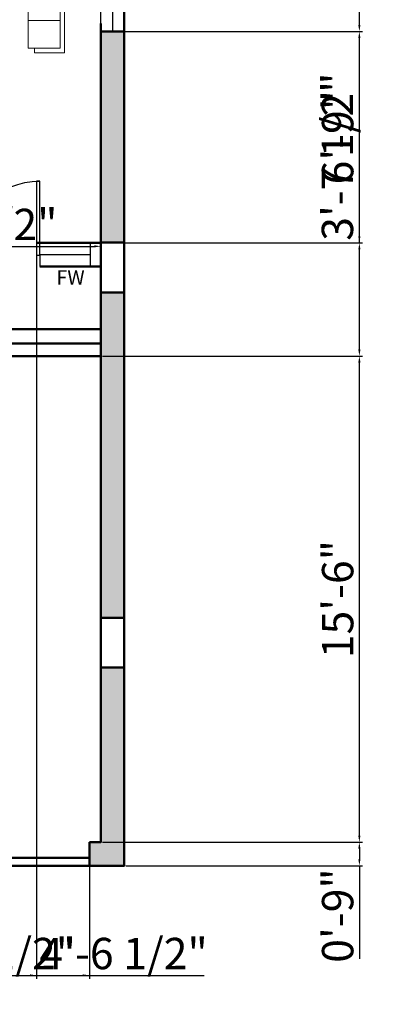
# Model space of a CAD drawing. Units: inches. Extents: x 2063 to 3370, y 2091 to 2971.
# Tile 2 of 14: x 2345 to 2486, y 2091 to 2468. Entities that reach past the tile are written whole.
import ezdxf

# ---------------------------------------------------------------- set-up
doc = ezdxf.new("R2010")
doc.units = ezdxf.units.IN
for name, color, linetype, lineweight in [('A-ANNO-DIMS', 2, 'Continuous', 18), ('A-ANNO-TEXT', 7, 'Continuous', 18), ('A-COLS', 7, 'Continuous', 50), ('A-DOOR', 4, 'Continuous', 25), ('A-FURN', 8, 'Continuous', 18), ('A-GLAZ', 131, 'Continuous', 25), ('A-WALL', 7, 'Continuous', 50), ('A-WALL-PATT', 8, 'Continuous', 13)]:
    doc.layers.add(name, color=color, linetype=linetype, lineweight=lineweight)
doc.styles.get("Standard").update_dxf_attribs({"font": 'arial.ttf'})
doc.dimstyles.new('ISO-25', dxfattribs={"dimtxt": 12, "dimasz": 2.5, "dimexe": 1.25, "dimexo": 0.625, "dimtad": 1, "dimdec": 0, "dimlunit": 4, "dimtxsty": 'Standard', "dimcen": 2.5, "dimadec": 0, "dimazin": 0, "dimtfac": 1, "dimtdec": 0, "dimtmove": 0, "dimatfit": 3, "dimfxl": 1, "dimarcsym": 0})

# ---------------------------------------------------------------- blocks, each defined once
blk = doc.blocks.new('*U2')
for p, q in [((0, 0), (0, -6)), ((40, 0), (40, -6))]:
    blk.add_line(p, q)
blk.add_lwpolyline([(0, 0), (0, 40), (1.75, 40), (1.75, 0)], close=True)
blk.add_arc((0, 0), 40, 0, 90)
blk = doc.blocks.new('SOFA-3SEAT')
for p, q in [((2.4, 33.13), (2.4, 35.12)), ((2.4, 35.12), (13.91, 35.12)), ((13.91, 35.12), (13.91, 0)), ((0, 23.31), (12.18, 23.31)), ((0, 12.42), (12.18, 12.42)), ((2.4, 0), (2.4, 1.81)), ((13.91, 0), (2.4, 0))]:
    blk.add_line(p, q)
blk.add_lwpolyline([(12.18, 33.13), (0, 33.13), (0, 1.81), (12.18, 1.81)], close=True)
blk = doc.blocks.new('*D41')
at = {"layer": 'A-ANNO-DIMS', "color": 0, "lineweight": -2, "transparency": 16777216}
for p, q in [((2296.75, 2152.8), (2296.75, 2101.18)), ((2371.36, 2152.8), (2371.36, 2101.18)), ((2299.25, 2102.43), (2368.86, 2102.43))]:
    blk.add_line(p, q, dxfattribs=at)
at = {"layer": 'A-ANNO-DIMS', "color": 0, "transparency": 16777216}
for points in [[(2299.25, 2102.84), (2299.25, 2102.01), (2296.75, 2102.43)], [(2368.86, 2102.84), (2368.86, 2102.01), (2371.36, 2102.43)]]:
    blk.add_solid(points, dxfattribs=at)
at = {"layer": 'Defpoints', "color": 0, "transparency": 16777216}
for p in [(2296.75, 2153.43), (2371.36, 2153.43), (2371.36, 2102.43)]:
    blk.add_point(p, dxfattribs=at)
at = {"layer": 'A-ANNO-DIMS', "color": 0, "transparency": 16777216, "insert": (2334.06, 2109.26), "char_height": 12, "attachment_point": 5}
blk.add_mtext('6\'-2 1/2"', dxfattribs=at)
blk = doc.blocks.new('*D43')
at = {"layer": 'A-ANNO-DIMS', "color": 0, "lineweight": -2, "transparency": 16777216}
for p, q in [((2278.17, 2340.25), (2278.17, 2382.88)), ((2280.67, 2381.63), (2373.22, 2381.63)), ((2375.72, 2340.25), (2375.72, 2382.88))]:
    blk.add_line(p, q, dxfattribs=at)
at = {"layer": 'A-ANNO-DIMS', "color": 0, "transparency": 16777216}
for points in [[(2280.67, 2382.04), (2280.67, 2381.21), (2278.17, 2381.63)], [(2373.22, 2382.04), (2373.22, 2381.21), (2375.72, 2381.63)]]:
    blk.add_solid(points, dxfattribs=at)
at = {"layer": 'Defpoints', "color": 0, "transparency": 16777216}
for p in [(2375.72, 2381.63), (2278.17, 2339.63), (2375.72, 2339.63)]:
    blk.add_point(p, dxfattribs=at)
at = {"layer": 'A-ANNO-DIMS', "color": 0, "transparency": 16777216, "insert": (2326.95, 2388.46), "char_height": 12, "attachment_point": 5}
blk.add_mtext('8\'-1 1/2"', dxfattribs=at)
blk = doc.blocks.new('*D46')
at = {"layer": 'A-ANNO-DIMS', "color": 0, "lineweight": -2, "transparency": 16777216}
for p, q in [((2296.8, 2382.3), (2296.8, 2101.18)), ((2351.15, 2382.3), (2351.15, 2101.18)), ((2299.3, 2102.43), (2348.65, 2102.43)), ((2351.15, 2102.43), (2415.24, 2102.43))]:
    blk.add_line(p, q, dxfattribs=at)
at = {"layer": 'A-ANNO-DIMS', "color": 0, "transparency": 16777216}
for points in [[(2299.3, 2102.84), (2299.3, 2102.01), (2296.8, 2102.43)], [(2348.65, 2102.84), (2348.65, 2102.01), (2351.15, 2102.43)]]:
    blk.add_solid(points, dxfattribs=at)
at = {"layer": 'Defpoints', "color": 0, "transparency": 16777216}
for p in [(2296.8, 2382.93), (2351.15, 2382.93), (2351.15, 2102.43)]:
    blk.add_point(p, dxfattribs=at)
at = {"layer": 'A-ANNO-DIMS', "color": 0, "transparency": 16777216, "insert": (2384.45, 2109.26), "char_height": 12, "attachment_point": 5}
blk.add_mtext('4\'-6 1/2"', dxfattribs=at)
blk = doc.blocks.new('*D59')
at = {"layer": 'A-ANNO-DIMS', "color": 0, "lineweight": -2, "transparency": 16777216}
for p, q in [((2376.35, 2153.43), (2475.9, 2153.43)), ((2474.65, 2150.93), (2474.65, 2146.93)), ((2385.35, 2144.43), (2475.9, 2144.43)), ((2474.65, 2144.43), (2474.65, 2108.78))]:
    blk.add_line(p, q, dxfattribs=at)
at = {"layer": 'A-ANNO-DIMS', "color": 0, "transparency": 16777216}
for points in [[(2474.23, 2150.93), (2475.06, 2150.93), (2474.65, 2153.43)], [(2474.23, 2146.93), (2475.06, 2146.93), (2474.65, 2144.43)]]:
    blk.add_solid(points, dxfattribs=at)
at = {"layer": 'Defpoints', "color": 0, "transparency": 16777216}
for p in [(2375.72, 2153.43), (2384.72, 2144.43), (2474.65, 2144.43)]:
    blk.add_point(p, dxfattribs=at)
at = {"layer": 'A-ANNO-DIMS', "color": 0, "transparency": 16777216, "insert": (2467.89, 2125.35), "char_height": 12, "attachment_point": 5, "rotation": 90}
blk.add_mtext('0\'-9"', dxfattribs=at)
blk = doc.blocks.new('*D60')
at = {"layer": 'A-ANNO-DIMS', "color": 0, "lineweight": -2, "transparency": 16777216}
for p, q in [((2376.35, 2339.63), (2475.9, 2339.63)), ((2474.65, 2155.93), (2474.65, 2337.13)), ((2376.35, 2153.43), (2475.9, 2153.43))]:
    blk.add_line(p, q, dxfattribs=at)
at = {"layer": 'A-ANNO-DIMS', "color": 0, "transparency": 16777216}
for points in [[(2474.23, 2337.13), (2475.06, 2337.13), (2474.65, 2339.63)], [(2474.23, 2155.93), (2475.06, 2155.93), (2474.65, 2153.43)]]:
    blk.add_solid(points, dxfattribs=at)
at = {"layer": 'Defpoints', "color": 0, "transparency": 16777216}
for p in [(2375.72, 2339.63), (2474.65, 2339.63), (2375.72, 2153.43)]:
    blk.add_point(p, dxfattribs=at)
at = {"layer": 'A-ANNO-DIMS', "color": 0, "transparency": 16777216, "insert": (2467.89, 2246.53), "char_height": 12, "attachment_point": 5, "rotation": 90}
blk.add_mtext('15\'-6"', dxfattribs=at)
blk = doc.blocks.new('*D61')
at = {"layer": 'A-ANNO-DIMS', "color": 0, "lineweight": -2, "transparency": 16777216}
for p, q in [((2474.65, 2382.93), (2474.65, 2446.53)), ((2376.35, 2382.93), (2475.9, 2382.93)), ((2474.65, 2342.13), (2474.65, 2380.43)), ((2376.35, 2339.63), (2475.9, 2339.63))]:
    blk.add_line(p, q, dxfattribs=at)
at = {"layer": 'A-ANNO-DIMS', "color": 0, "transparency": 16777216}
for points in [[(2474.23, 2380.43), (2475.06, 2380.43), (2474.65, 2382.93)], [(2474.23, 2342.13), (2475.06, 2342.13), (2474.65, 2339.63)]]:
    blk.add_solid(points, dxfattribs=at)
at = {"layer": 'Defpoints', "color": 0, "transparency": 16777216}
for p in [(2375.72, 2382.93), (2474.65, 2382.93), (2375.72, 2339.63)]:
    blk.add_point(p, dxfattribs=at)
at = {"layer": 'A-ANNO-DIMS', "color": 0, "transparency": 16777216, "insert": (2467.81, 2415.98), "char_height": 12, "attachment_point": 5, "rotation": 90}
blk.add_mtext('3\'-7 1/2"', dxfattribs=at)
blk = doc.blocks.new('*D62')
at = {"layer": 'A-ANNO-DIMS', "color": 0, "lineweight": -2, "transparency": 16777216}
for p, q in [((2376.35, 2463.93), (2475.9, 2463.93)), ((2474.65, 2385.43), (2474.65, 2461.43)), ((2376.35, 2382.93), (2475.9, 2382.93))]:
    blk.add_line(p, q, dxfattribs=at)
at = {"layer": 'A-ANNO-DIMS', "color": 0, "transparency": 16777216}
for points in [[(2474.23, 2461.43), (2475.06, 2461.43), (2474.65, 2463.93)], [(2474.23, 2385.43), (2475.06, 2385.43), (2474.65, 2382.93)]]:
    blk.add_solid(points, dxfattribs=at)
at = {"layer": 'Defpoints', "color": 0, "transparency": 16777216}
for p in [(2375.72, 2463.93), (2474.65, 2463.93), (2375.72, 2382.93)]:
    blk.add_point(p, dxfattribs=at)
at = {"layer": 'A-ANNO-DIMS', "color": 0, "transparency": 16777216, "insert": (2467.89, 2423.43), "char_height": 12, "attachment_point": 5, "rotation": 90}
blk.add_mtext('6\'-9"', dxfattribs=at)
blk = doc.blocks.new('*D63')
at = {"layer": 'A-ANNO-DIMS', "color": 0, "lineweight": -2, "transparency": 16777216}
for p, q in [((2376.35, 2523.93), (2475.9, 2523.93)), ((2474.65, 2466.43), (2474.65, 2521.43)), ((2376.35, 2463.93), (2475.9, 2463.93))]:
    blk.add_line(p, q, dxfattribs=at)
at = {"layer": 'A-ANNO-DIMS', "color": 0, "transparency": 16777216}
for points in [[(2474.23, 2521.43), (2475.06, 2521.43), (2474.65, 2523.93)], [(2474.23, 2466.43), (2475.06, 2466.43), (2474.65, 2463.93)]]:
    blk.add_solid(points, dxfattribs=at)
at = {"layer": 'Defpoints', "color": 0, "transparency": 16777216}
for p in [(2375.72, 2523.93), (2474.65, 2523.93), (2375.72, 2463.93)]:
    blk.add_point(p, dxfattribs=at)
at = {"layer": 'A-ANNO-DIMS', "color": 0, "transparency": 16777216, "insert": (2467.89, 2493.93), "char_height": 12, "attachment_point": 5, "rotation": 90}
blk.add_mtext('5\'-0"', dxfattribs=at)

msp = doc.modelspace()

# ---------------------------------------------------------------- hatches: boundary and pattern name
at = {"layer": 'A-WALL-PATT'}
h = msp.add_hatch(color=256, dxfattribs=at)
h.dxf.hatch_style = 1
h.paths.add_polyline_path([(2384.72, 2679.03), (2375.72, 2679.03), (2375.72, 2645.28), (2384.72, 2645.28)])
h.paths.add_polyline_path([(2384.72, 2626.16), (2375.72, 2626.16), (2375.72, 2576.43), (2327.14, 2576.43), (2327.14, 2571.93), (2375.72, 2571.93), (2375.72, 2523.93), (2384.72, 2523.93)])
h.paths.add_polyline_path([(2384.72, 2463.93), (2375.72, 2463.93), (2375.72, 2383.04), (2384.72, 2383.04)])
h.paths.add_polyline_path([(2153.72, 2812.31), (2144.72, 2812.31), (2144.72, 2638.63), (2153.72, 2638.63)])
h.paths.add_polyline_path([(2225.08, 2576.43), (2153.72, 2576.43), (2153.72, 2619.52), (2144.72, 2619.52), (2144.72, 2420.38), (2153.72, 2420.38), (2153.72, 2466.93), (2175.31, 2466.93), (2175.31, 2471.43), (2153.72, 2471.43), (2153.72, 2519.43), (2213.72, 2519.43), (2213.72, 2507.47), (2214.09, 2507.47), (2218.22, 2507.47), (2218.22, 2519.43), (2218.22, 2523.93), (2218.22, 2529.53), (2213.72, 2529.53), (2213.72, 2523.93), (2153.72, 2523.93), (2153.72, 2571.93), (2213.72, 2571.93), (2213.72, 2563.16), (2218.22, 2563.16), (2218.22, 2571.93), (2225.08, 2571.93)])
h = msp.add_hatch(color=256, dxfattribs=at)
h.dxf.hatch_style = 1
h.paths.add_polyline_path([(2153.72, 2222.57), (2144.72, 2222.57), (2144.72, 2144.43), (2296.75, 2144.43), (2296.75, 2153.43), (2153.72, 2153.43)])
h.paths.add_polyline_path([(2384.72, 2220.3), (2375.72, 2220.3), (2375.72, 2153.43), (2371.36, 2153.43), (2371.36, 2144.43), (2384.72, 2144.43)])
h.paths.add_polyline_path([(2384.72, 2363.93), (2375.72, 2363.93), (2375.72, 2239.41), (2384.72, 2239.41)])
h.paths.add_polyline_path([(2153.72, 2396.38), (2144.72, 2396.38), (2144.72, 2382.93), (2153.72, 2382.93)])

# ---------------------------------------------------------------- linework, layer by layer
at = {"layer": 'A-COLS'}
for points in [[(2375.72, 2383.04), (2384.72, 2383.04), (2384.72, 2363.93), (2375.72, 2363.93)], [(2375.72, 2239.41), (2384.72, 2239.41), (2384.72, 2220.3), (2375.72, 2220.3)]]:
    msp.add_lwpolyline(points, close=True, dxfattribs=at)
at = {"layer": 'A-GLAZ'}
for p, q in [((2375.72, 2466.93), (2375.72, 2523.93)), ((2380.22, 2523.93), (2380.22, 2463.93)), ((2371.67, 2382.93), (2371.67, 2373.93)), ((2371.67, 2378.43), (2352.39, 2378.43))]:
    msp.add_line(p, q, dxfattribs=at)
at = {"layer": 'A-WALL'}
for p, q in [((2375.72, 2463.93), (2384.72, 2463.93)), ((2351.15, 2382.93), (2375.72, 2382.93)), ((2352.39, 2373.93), (2375.72, 2373.93)), ((2278.17, 2349.93), (2374.17, 2349.93)), ((2374.17, 2349.93), (2375.72, 2349.93)), ((2278.17, 2344.41), (2374.17, 2344.41)), ((2374.17, 2344.41), (2375.72, 2344.41)), ((2278.17, 2339.63), (2374.17, 2339.63)), ((2374.17, 2339.63), (2375.72, 2339.63)), ((2371.36, 2153.43), (2371.36, 2144.43)), ((2371.36, 2153.43), (2371.36, 2144.43))]:
    msp.add_line(p, q, dxfattribs=at)
for points in [[(2144.72, 2144.43), (2384.72, 2144.43), (2384.72, 2864.43), (2144.72, 2864.43)], [(2296.75, 2144.43), (2371.36, 2144.43), (2371.36, 2147.44), (2296.75, 2147.44)]]:
    msp.add_lwpolyline(points, close=True, dxfattribs=at)
for points in [[(2375.72, 2382.93), (2375.72, 2466.93)], [(2375.72, 2234.43), (2375.72, 2378.43)], [(2371.36, 2153.43), (2375.72, 2153.43), (2375.72, 2225.43)]]:
    msp.add_lwpolyline(points, dxfattribs=at)

# ---------------------------------------------------------------- block references
at = {"layer": 'A-DOOR', "xscale": -0.7105099264086059, "yscale": 0.7105099264086059, "zscale": 0.7105099264086059}
msp.add_blockref('*U2', (2352.39, 2378.19), dxfattribs=at)
at = {"layer": 'A-FURN'}
msp.add_blockref('SOFA-3SEAT', (2347.98, 2455.72), dxfattribs=at)

# ---------------------------------------------------------------- texts
at = {"layer": 'A-ANNO-TEXT', "insert": (2358.78, 2372.47), "char_height": 5.523, "attachment_point": 1}
msp.add_mtext_dynamic_manual_height_columns('FW', width=106.0361, gutter_width=27.61, heights=[0], dxfattribs=at)

# ---------------------------------------------------------------- dimensions: what is measured, and where the dimension line sits
at = {"layer": 'A-ANNO-DIMS'}
for base, p1, p2, picture, middle in [((2474.65, 2523.93), (2375.72, 2463.93), (2375.72, 2523.93), '*D63', (2467.89, 2493.93)), ((2474.65, 2463.93), (2375.72, 2382.93), (2375.72, 2463.93), '*D62', (2467.89, 2423.43)), ((2474.65, 2382.93), (2375.72, 2339.63), (2375.72, 2382.93), '*D61', (2467.81, 2415.98)), ((2474.65, 2339.63), (2375.72, 2153.43), (2375.72, 2339.63), '*D60', (2467.89, 2246.53)), ((2474.65, 2144.43), (2375.72, 2153.43), (2384.72, 2144.43), '*D59', (2467.89, 2125.35))]:
    dim = msp.add_linear_dim(base=base, p1=p1, p2=p2, angle=90, dimstyle='ISO-25', override={"dimdec": 1, "dimlfac": 1, "dimrnd": 0, "dimzin": 1, "dimdsep": 46, "dimlunit": 4, "dimfrac": 2}, dxfattribs=at)
    dim.commit()
    dim.dimension.update_dxf_attribs({"geometry": picture, "text_midpoint": middle})
for base, p1, p2, picture, middle in [((2375.722, 2381.628), (2278.1707, 2339.628), (2375.722, 2339.628), '*D43', (2326.9464, 2388.4576)), ((2351.1508, 2102.4264), (2296.7967, 2382.9264), (2351.1508, 2382.9264), '*D46', (2384.4476, 2109.2561)), ((2371.36, 2102.43), (2296.75, 2153.43), (2371.36, 2153.43), '*D41', (2334.06, 2109.26))]:
    dim = msp.add_linear_dim(base=base, p1=p1, p2=p2, dimstyle='ISO-25', override={"dimdec": 1, "dimlfac": 1, "dimrnd": 0, "dimzin": 1, "dimdsep": 46, "dimlunit": 4, "dimfrac": 2}, dxfattribs=at)
    dim.commit()
    dim.dimension.update_dxf_attribs({"geometry": picture, "text_midpoint": middle})

doc.saveas('drawing.dxf')
